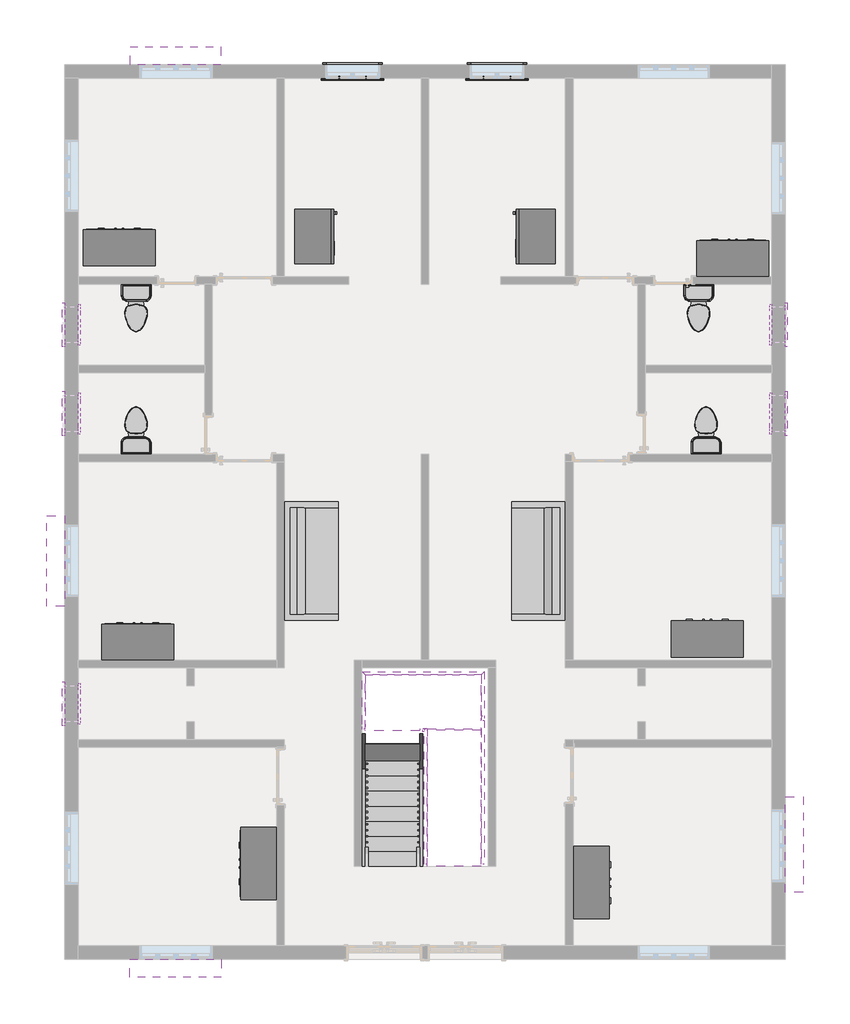
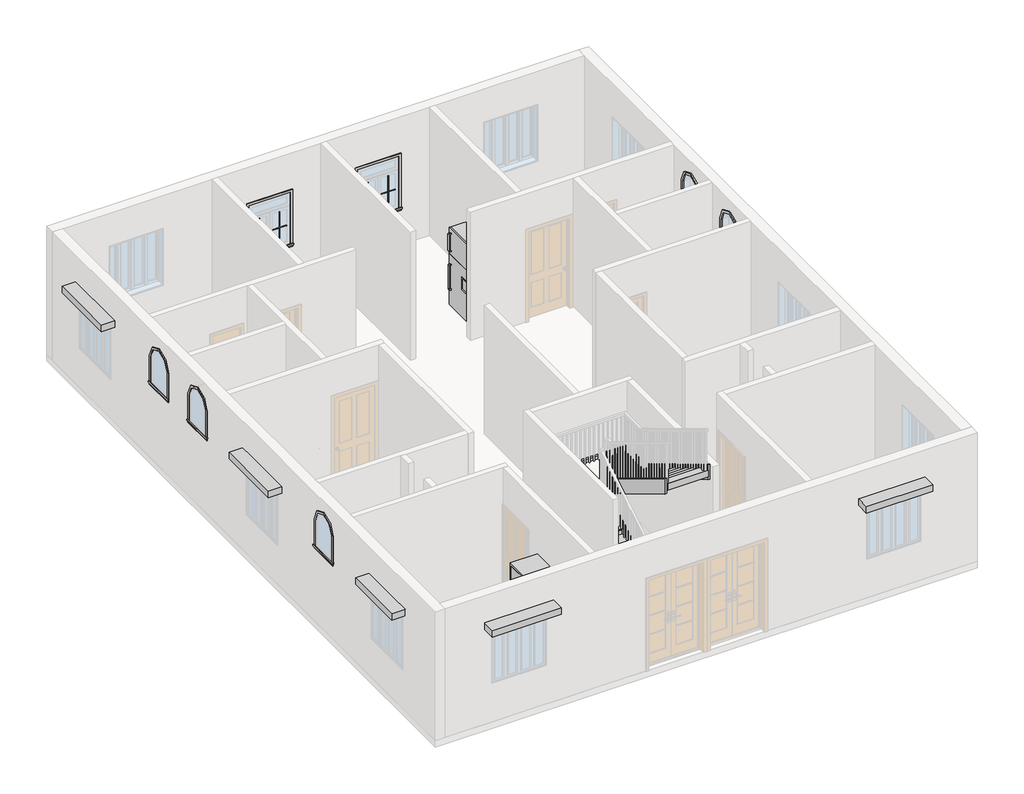
# One storey, part 4 of 4: 22 proxies, 10 furniture elements, 8 members, 4 flow terminals, 2 stair flights, 1 slab.
"""IFC4 building model written with IfcOpenShell, lengths in millimetres."""

from ifc_helpers import new_model, si_unit, frame, origin, place, context, project, spatial, polyline, outline, extrude, faceted_brep, transform, mapped, element, save
from components import generic_models_1_generic_models_1_2a4bce15, generic_models_2_generic_models_2_71c639ae, generic_models_3_generic_models_3_01e5b337, generic_models_4_generic_models_4_21550f0b, muntin_pattern_2x2_muntin_pattern_2x2_d1c6e638, muntin_pattern_2x2_muntin_pattern_2x2_37b95fb2, trim_window_exterior_flat_with_sill_80371c4b, trim_window_exterior_flat_arch_top_tree_centered_with_sill_b3d54518, trim_window_interior_flat_picture_frame_c1dcbb6d, trim_window_interior_flat_arch_top_tree_centered_picture_1d59b3d4, toilet_domestic_3d_toilet_domestic_3d_ba6479b0, toilet_domestic_3d_toilet_domestic_3d_30431060, furniture_65fa61b5, furniture_3f4f9d7a, furniture_123_or_4_seats_couch_4554_e45b83ba, furniture_82e269c4, non_monolithic_landing_68493687, stair_flight_7beec1f7, stair_flight_0e2f1c24

model = new_model("IFC4")

# Units and contexts
model_context = context("Model", 3, world=origin())
ifc_project = project(units=[si_unit("LENGTHUNIT", "METRE", prefix="MILLI")], contexts=[model_context])

# Site, building, storey
site = spatial("IfcSite", under=ifc_project)
building = spatial("IfcBuilding", under=site)
storey = spatial("IfcBuildingStorey", under=building, Elevation=0.0)

# Proxies
placement = place(None, origin())
generic_models_1_generic_models_1_shape = generic_models_1_generic_models_1_2a4bce15(model_context)
element("IfcBuildingElementProxy", 1, Name="Generic Models 1 : Generic Models 1", ObjectType="Generic Models 1 : Generic Models 1", at=placement, inside=storey, context=model_context, shape_type="MappedRepresentation", body=[
    mapped(generic_models_1_generic_models_1_shape, transform((0.0, 0.0, 0.0), x_axis=(1.0, 0.0, 0.0), y_axis=(0.0, 1.0, 0.0), z_axis=(0.0, 0.0, 1.0))),
])
generic_models_2_generic_models_2_shape = generic_models_2_generic_models_2_71c639ae(model_context)
element("IfcBuildingElementProxy", 2, Name="Generic Models 2 : Generic Models 2", ObjectType="Generic Models 2 : Generic Models 2", at=placement, inside=storey, context=model_context, shape_type="MappedRepresentation", body=[
    mapped(generic_models_2_generic_models_2_shape, transform((0.0, 0.0, 0.0), x_axis=(1.0, 0.0, 0.0), y_axis=(0.0, 1.0, 0.0), z_axis=(0.0, 0.0, 1.0))),
])
generic_models_3_generic_models_3_shape = generic_models_3_generic_models_3_01e5b337(model_context)
element("IfcBuildingElementProxy", 3, Name="Generic Models 3 : Generic Models 3", ObjectType="Generic Models 3 : Generic Models 3", at=placement, inside=storey, context=model_context, shape_type="MappedRepresentation", body=[
    mapped(generic_models_3_generic_models_3_shape, transform((0.0, 0.0, 0.0), x_axis=(1.0, 0.0, 0.0), y_axis=(0.0, 1.0, 0.0), z_axis=(0.0, 0.0, 1.0))),
])
generic_models_4_generic_models_4_shape = generic_models_4_generic_models_4_21550f0b(model_context)
element("IfcBuildingElementProxy", 4, Name="Generic Models 4 : Generic Models 4", ObjectType="Generic Models 4 : Generic Models 4", at=placement, inside=storey, context=model_context, shape_type="MappedRepresentation", body=[
    mapped(generic_models_4_generic_models_4_shape, transform((0.0, 0.0, 0.0), x_axis=(1.0, 0.0, 0.0), y_axis=(0.0, 1.0, 0.0), z_axis=(0.0, 0.0, 1.0))),
])
muntin_pattern_2x2_muntin_pattern_2x2_shape = muntin_pattern_2x2_muntin_pattern_2x2_d1c6e638(model_context)
element("IfcBuildingElementProxy", 5, Name="Muntin Pattern_2x2 : Muntin Pattern_2x2", ObjectType="Muntin Pattern_2x2 : Muntin Pattern_2x2", at=placement, inside=storey, context=model_context, shape_type="MappedRepresentation", body=[
    mapped(muntin_pattern_2x2_muntin_pattern_2x2_shape, transform((-10531.1646954, 8361.6522103, 984.25), x_axis=(-1.0, 0.0, 0.0), y_axis=(0.0, -1.0, 0.0), z_axis=(0.0, 0.0, 1.0))),
])
element("IfcBuildingElementProxy", 6, Name="Muntin Pattern_2x2 : Muntin Pattern_2x2", ObjectType="Muntin Pattern_2x2 : Muntin Pattern_2x2", at=placement, inside=storey, context=model_context, shape_type="MappedRepresentation", body=[
    mapped(muntin_pattern_2x2_muntin_pattern_2x2_shape, transform((-8092.7646954, 8361.6522103, 984.25), x_axis=(-1.0, 0.0, 0.0), y_axis=(0.0, -1.0, 0.0), z_axis=(0.0, 0.0, 1.0))),
])
muntin_pattern_2x2_muntin_pattern_2x2_2_shape = muntin_pattern_2x2_muntin_pattern_2x2_37b95fb2(model_context)
element("IfcBuildingElementProxy", 7, Name="Muntin Pattern_2x2 : Muntin Pattern_2x2", ObjectType="Muntin Pattern_2x2 : Muntin Pattern_2x2", at=placement, inside=storey, context=model_context, shape_type="MappedRepresentation", body=[
    mapped(muntin_pattern_2x2_muntin_pattern_2x2_2_shape, transform((-10985.1896954, 8361.6522103, 984.25), x_axis=(1.0, 0.0, 0.0), y_axis=(0.0, 1.0, 0.0), z_axis=(0.0, 0.0, 1.0))),
])
element("IfcBuildingElementProxy", 8, Name="Muntin Pattern_2x2 : Muntin Pattern_2x2", ObjectType="Muntin Pattern_2x2 : Muntin Pattern_2x2", at=placement, inside=storey, context=model_context, shape_type="MappedRepresentation", body=[
    mapped(muntin_pattern_2x2_muntin_pattern_2x2_2_shape, transform((-8546.7896954, 8361.6522103, 984.25), x_axis=(1.0, 0.0, 0.0), y_axis=(0.0, 1.0, 0.0), z_axis=(0.0, 0.0, 1.0))),
])
trim_window_exterior_flat_with_sill_shape = trim_window_exterior_flat_with_sill_80371c4b(model_context)
element("IfcBuildingElementProxy", 9, Name="Trim-Window-Exterior-Flat : with Sill", ObjectType="Trim-Window-Exterior-Flat : with Sill", at=placement, inside=storey, context=model_context, shape_type="MappedRepresentation", body=[
    mapped(trim_window_exterior_flat_with_sill_shape, transform((-10758.1771954, 8352.1272103, 2133.6), x_axis=(-1.0, 0.0, 0.0), y_axis=(0.0, 0.0, -1.0), z_axis=(0.0, -1.0, 0.0))),
])
element("IfcBuildingElementProxy", 10, Name="Trim-Window-Exterior-Flat : with Sill", ObjectType="Trim-Window-Exterior-Flat : with Sill", at=placement, inside=storey, context=model_context, shape_type="MappedRepresentation", body=[
    mapped(trim_window_exterior_flat_with_sill_shape, transform((-8319.7771954, 8352.1272103, 2133.6), x_axis=(-1.0, 0.0, 0.0), y_axis=(0.0, 0.0, -1.0), z_axis=(0.0, -1.0, 0.0))),
])
trim_window_exterior_flat_arch_top_tree_centered_with_sill_shape = trim_window_exterior_flat_arch_top_tree_centered_with_sill_b3d54518(model_context)
element("IfcBuildingElementProxy", 11, Name="Trim-Window-Exterior-Flat-Arch-Top-Tree_Centered : with Sill", ObjectType="Trim-Window-Exterior-Flat-Arch-Top-Tree_Centered : with Sill", at=placement, inside=storey, context=model_context, shape_type="MappedRepresentation", body=[
    mapped(trim_window_exterior_flat_arch_top_tree_centered_with_sill_shape, transform((-15623.8646954, -2214.2727897, 2743.2), x_axis=(0.0, -1.0, 0.0), y_axis=(0.0, 0.0, 1.0), z_axis=(-1.0, 0.0, 0.0))),
])
element("IfcBuildingElementProxy", 12, Name="Trim-Window-Exterior-Flat-Arch-Top-Tree_Centered : with Sill", ObjectType="Trim-Window-Exterior-Flat-Arch-Top-Tree_Centered : with Sill", at=placement, inside=storey, context=model_context, shape_type="MappedRepresentation", body=[
    mapped(trim_window_exterior_flat_arch_top_tree_centered_with_sill_shape, transform((-3455.6771954, 2688.1919086, 2743.2), x_axis=(0.0, 1.0, 0.0), y_axis=(0.0, 0.0, 1.0), z_axis=(1.0, 0.0, 0.0))),
])
element("IfcBuildingElementProxy", 13, Name="Trim-Window-Exterior-Flat-Arch-Top-Tree_Centered : with Sill", ObjectType="Trim-Window-Exterior-Flat-Arch-Top-Tree_Centered : with Sill", at=placement, inside=storey, context=model_context, shape_type="MappedRepresentation", body=[
    mapped(trim_window_exterior_flat_arch_top_tree_centered_with_sill_shape, transform((-3455.6771954, 4186.5272103, 2743.2), x_axis=(0.0, 1.0, 0.0), y_axis=(0.0, 0.0, 1.0), z_axis=(1.0, 0.0, 0.0))),
])
element("IfcBuildingElementProxy", 14, Name="Trim-Window-Exterior-Flat-Arch-Top-Tree_Centered : with Sill", ObjectType="Trim-Window-Exterior-Flat-Arch-Top-Tree_Centered : with Sill", at=placement, inside=storey, context=model_context, shape_type="MappedRepresentation", body=[
    mapped(trim_window_exterior_flat_arch_top_tree_centered_with_sill_shape, transform((-15623.8646954, 2688.1919086, 2743.2), x_axis=(0.0, -1.0, 0.0), y_axis=(0.0, 0.0, 1.0), z_axis=(-1.0, 0.0, 0.0))),
])
element("IfcBuildingElementProxy", 15, Name="Trim-Window-Exterior-Flat-Arch-Top-Tree_Centered : with Sill", ObjectType="Trim-Window-Exterior-Flat-Arch-Top-Tree_Centered : with Sill", at=placement, inside=storey, context=model_context, shape_type="MappedRepresentation", body=[
    mapped(trim_window_exterior_flat_arch_top_tree_centered_with_sill_shape, transform((-15623.8646954, 4186.5272103, 2743.2), x_axis=(0.0, -1.0, 0.0), y_axis=(0.0, 0.0, 1.0), z_axis=(-1.0, 0.0, 0.0))),
])
trim_window_interior_flat_picture_frame_shape = trim_window_interior_flat_picture_frame_c1dcbb6d(model_context)
element("IfcBuildingElementProxy", 16, Name="Trim-Window-Interior-Flat : Picture Frame", ObjectType="Trim-Window-Interior-Flat : Picture Frame", at=placement, inside=storey, context=model_context, shape_type="MappedRepresentation", body=[
    mapped(trim_window_interior_flat_picture_frame_shape, transform((-10758.1771954, 8580.7272103, 2133.6), x_axis=(1.0, 0.0, 0.0), y_axis=(0.0, 0.0, -1.0), z_axis=(0.0, 1.0, 0.0))),
])
element("IfcBuildingElementProxy", 17, Name="Trim-Window-Interior-Flat : Picture Frame", ObjectType="Trim-Window-Interior-Flat : Picture Frame", at=placement, inside=storey, context=model_context, shape_type="MappedRepresentation", body=[
    mapped(trim_window_interior_flat_picture_frame_shape, transform((-8319.7771954, 8580.7272103, 2133.6), x_axis=(1.0, 0.0, 0.0), y_axis=(0.0, 0.0, -1.0), z_axis=(0.0, 1.0, 0.0))),
])
trim_window_interior_flat_arch_top_tree_centered_picture_shape = trim_window_interior_flat_arch_top_tree_centered_picture_1d59b3d4(model_context)
element("IfcBuildingElementProxy", 18, Name="Trim-Window-Interior-Flat-Arch-Top-Tree_Centered : Picture Frame", ObjectType="Trim-Window-Interior-Flat-Arch-Top-Tree_Centered : Picture Frame", at=placement, inside=storey, context=model_context, shape_type="MappedRepresentation", body=[
    mapped(trim_window_interior_flat_arch_top_tree_centered_picture_shape, transform((-15395.2646954, -2214.2727897, 2743.2), x_axis=(0.0, 1.0, 0.0), y_axis=(0.0, 0.0, 1.0), z_axis=(1.0, 0.0, 0.0))),
])
element("IfcBuildingElementProxy", 19, Name="Trim-Window-Interior-Flat-Arch-Top-Tree_Centered : Picture Frame", ObjectType="Trim-Window-Interior-Flat-Arch-Top-Tree_Centered : Picture Frame", at=placement, inside=storey, context=model_context, shape_type="MappedRepresentation", body=[
    mapped(trim_window_interior_flat_arch_top_tree_centered_picture_shape, transform((-3684.2771954, 2688.1919086, 2743.2), x_axis=(0.0, -1.0, 0.0), y_axis=(0.0, 0.0, 1.0), z_axis=(-1.0, 0.0, 0.0))),
])
element("IfcBuildingElementProxy", 20, Name="Trim-Window-Interior-Flat-Arch-Top-Tree_Centered : Picture Frame", ObjectType="Trim-Window-Interior-Flat-Arch-Top-Tree_Centered : Picture Frame", at=placement, inside=storey, context=model_context, shape_type="MappedRepresentation", body=[
    mapped(trim_window_interior_flat_arch_top_tree_centered_picture_shape, transform((-3684.2771954, 4186.5272103, 2743.2), x_axis=(0.0, -1.0, 0.0), y_axis=(0.0, 0.0, 1.0), z_axis=(-1.0, 0.0, 0.0))),
])
element("IfcBuildingElementProxy", 21, Name="Trim-Window-Interior-Flat-Arch-Top-Tree_Centered : Picture Frame", ObjectType="Trim-Window-Interior-Flat-Arch-Top-Tree_Centered : Picture Frame", at=placement, inside=storey, context=model_context, shape_type="MappedRepresentation", body=[
    mapped(trim_window_interior_flat_arch_top_tree_centered_picture_shape, transform((-15395.2646954, 2688.1919086, 2743.2), x_axis=(0.0, 1.0, 0.0), y_axis=(0.0, 0.0, 1.0), z_axis=(1.0, 0.0, 0.0))),
])
element("IfcBuildingElementProxy", 22, Name="Trim-Window-Interior-Flat-Arch-Top-Tree_Centered : Picture Frame", ObjectType="Trim-Window-Interior-Flat-Arch-Top-Tree_Centered : Picture Frame", at=placement, inside=storey, context=model_context, shape_type="MappedRepresentation", body=[
    mapped(trim_window_interior_flat_arch_top_tree_centered_picture_shape, transform((-15395.2646954, 4186.5272103, 2743.2), x_axis=(0.0, 1.0, 0.0), y_axis=(0.0, 0.0, 1.0), z_axis=(1.0, 0.0, 0.0))),
])

# Flow terminals
toilet_domestic_3d_toilet_domestic_3d_shape = toilet_domestic_3d_toilet_domestic_3d_ba6479b0(model_context)
toilet_domestic_3d_toilet_domestic_3d_2_shape = toilet_domestic_3d_toilet_domestic_3d_30431060(model_context)
element("IfcFlowTerminal", 23, ObjectType="Toilet-Domestic-3D : Toilet-Domestic-3D", at=placement, inside=storey, context=model_context, shape_type="MappedRepresentation", body=[
    mapped(toilet_domestic_3d_toilet_domestic_3d_shape, transform((-14415.7771954, 4377.631183, 0.0), x_axis=(1.0, 0.0, 0.0), y_axis=(0.0, 1.0, 0.0), z_axis=(0.0, 0.0, 1.0))),
    mapped(toilet_domestic_3d_toilet_domestic_3d_2_shape, transform((-14415.7771954, 4377.631183, 0.0), x_axis=(1.0, 0.0, 0.0), y_axis=(0.0, 1.0, 0.0), z_axis=(0.0, 0.0, 1.0))),
])
element("IfcFlowTerminal", 24, ObjectType="Toilet-Domestic-3D : Toilet-Domestic-3D", at=placement, inside=storey, context=model_context, shape_type="MappedRepresentation", body=[
    mapped(toilet_domestic_3d_toilet_domestic_3d_shape, transform((-14417.3646954, 2497.3526342, 0.0), x_axis=(-1.0, 0.0, 0.0), y_axis=(0.0, -1.0, 0.0), z_axis=(0.0, 0.0, 1.0))),
    mapped(toilet_domestic_3d_toilet_domestic_3d_2_shape, transform((-14417.3646954, 2497.3526342, 0.0), x_axis=(-1.0, 0.0, 0.0), y_axis=(0.0, -1.0, 0.0), z_axis=(0.0, 0.0, 1.0))),
])
element("IfcFlowTerminal", 25, ObjectType="Toilet-Domestic-3D : Toilet-Domestic-3D", at=placement, inside=storey, context=model_context, shape_type="MappedRepresentation", body=[
    mapped(toilet_domestic_3d_toilet_domestic_3d_shape, transform((-4789.1771954, 2497.3526342, 0.0), x_axis=(-1.0, 0.0, 0.0), y_axis=(0.0, -1.0, 0.0), z_axis=(0.0, 0.0, 1.0))),
    mapped(toilet_domestic_3d_toilet_domestic_3d_2_shape, transform((-4789.1771954, 2497.3526342, 0.0), x_axis=(-1.0, 0.0, 0.0), y_axis=(0.0, -1.0, 0.0), z_axis=(0.0, 0.0, 1.0))),
])
element("IfcFlowTerminal", 26, ObjectType="Toilet-Domestic-3D : Toilet-Domestic-3D", at=placement, inside=storey, context=model_context, shape_type="MappedRepresentation", body=[
    mapped(toilet_domestic_3d_toilet_domestic_3d_shape, transform((-4916.1771954, 4377.631183, 0.0), x_axis=(1.0, 0.0, 0.0), y_axis=(0.0, 1.0, 0.0), z_axis=(0.0, 0.0, 1.0))),
    mapped(toilet_domestic_3d_toilet_domestic_3d_2_shape, transform((-4916.1771954, 4377.631183, 0.0), x_axis=(1.0, 0.0, 0.0), y_axis=(0.0, 1.0, 0.0), z_axis=(0.0, 0.0, 1.0))),
])

# Furniture
furniture_shape = furniture_65fa61b5(model_context)
element("IfcFurniture", 27, at=placement, inside=storey, context=model_context, shape_type="MappedRepresentation", body=[
    mapped(furniture_shape, transform((-11740.80602, 6289.078474, 0.0), x_axis=(0.0, 1.0, 0.0), y_axis=(-1.0, 0.0, 0.0), z_axis=(0.0, 0.0, 1.0))),
])
furniture_2_shape = furniture_3f4f9d7a(model_context)
element("IfcFurniture", 28, at=placement, inside=storey, context=model_context, shape_type="MappedRepresentation", body=[
    mapped(furniture_2_shape, transform((-7338.7358708, 6289.078474, 0.0), x_axis=(0.0, 1.0, 0.0), y_axis=(-1.0, 0.0, 0.0), z_axis=(0.0, 0.0, 1.0))),
])
furniture_123_or_4_seats_couch_4554_shape = furniture_123_or_4_seats_couch_4554_e45b83ba(model_context)
element("IfcFurniture", 29, ObjectType="123_or_4_seats_couch_4554", at=placement, inside=storey, context=model_context, shape_type="MappedRepresentation", body=[
    mapped(furniture_123_or_4_seats_couch_4554_shape, transform((-11913.8771954, 122.7919086, 0.0), x_axis=(8.148770547222739e-11, 1.0, 0.0), y_axis=(-1.0, 8.148770547222739e-11, 0.0), z_axis=(0.0, 0.0, 1.0))),
])
element("IfcFurniture", 30, ObjectType="123_or_4_seats_couch_4554", at=placement, inside=storey, context=model_context, shape_type="MappedRepresentation", body=[
    mapped(furniture_123_or_4_seats_couch_4554_shape, transform((-7164.0771954, 275.1919086, 0.0), x_axis=(0.0, -1.0, 0.0), y_axis=(1.0, 0.0, 0.0), z_axis=(0.0, 0.0, 1.0))),
])
furniture_3_shape = furniture_82e269c4(model_context)
element("IfcFurniture", 31, ObjectType="Wardrobe : 48\" x 72\" x 24\"", at=placement, inside=storey, context=model_context, shape_type="MappedRepresentation", body=[
    mapped(furniture_3_shape, transform((-14969.1544857, 4905.0525787, 0.0), x_axis=(-1.0, 0.0, 0.0), y_axis=(0.0, -1.0, 0.0), z_axis=(0.0, 0.0, 1.0))),
])
element("IfcFurniture", 32, ObjectType="Wardrobe : 48\" x 72\" x 24\"", at=placement, inside=storey, context=model_context, shape_type="MappedRepresentation", body=[
    mapped(furniture_3_shape, transform((-4609.4240791, 4720.3884008, 0.0), x_axis=(-1.0, 0.0, 0.0), y_axis=(0.0, -1.0, 0.0), z_axis=(0.0, 0.0, 1.0))),
])
element("IfcFurniture", 33, ObjectType="Wardrobe : 48\" x 72\" x 24\"", at=placement, inside=storey, context=model_context, shape_type="MappedRepresentation", body=[
    mapped(furniture_3_shape, transform((-14654.9354475, -1756.6115992, 0.0), x_axis=(-1.0, 0.0, 0.0), y_axis=(0.0, -1.0, 0.0), z_axis=(0.0, 0.0, 1.0))),
])
element("IfcFurniture", 34, ObjectType="Wardrobe : 48\" x 72\" x 24\"", at=placement, inside=storey, context=model_context, shape_type="MappedRepresentation", body=[
    mapped(furniture_3_shape, transform((-5037.6875981, -1704.33178, 0.0), x_axis=(-1.0, 0.0, 0.0), y_axis=(0.0, -1.0, 0.0), z_axis=(0.0, 0.0, 1.0))),
])
element("IfcFurniture", 35, ObjectType="Wardrobe : 48\" x 72\" x 24\"", at=placement, inside=storey, context=model_context, shape_type="MappedRepresentation", body=[
    mapped(furniture_3_shape, transform((-7316.016005, -4965.0574511, 0.0), x_axis=(0.0, 1.0, 0.0), y_axis=(-1.0, 0.0, 0.0), z_axis=(0.0, 0.0, 1.0))),
])
element("IfcFurniture", 36, ObjectType="Wardrobe : 48\" x 72\" x 24\"", at=placement, inside=storey, context=model_context, shape_type="MappedRepresentation", body=[
    mapped(furniture_3_shape, transform((-11761.9383858, -5181.4279362, 0.0), x_axis=(0.0, -1.0, 0.0), y_axis=(1.0, 0.0, 0.0), z_axis=(0.0, 0.0, 1.0))),
])

# Members
element("IfcMember", 37, ObjectType="Stringer - 2\" Width", at=placement, inside=storey, context=model_context, shape_type="SweptSolid", body=[
    extrude(outline(polyline([(-4957.4727897, 0.0), (-4957.4727897, 211.5517384), (-2643.0590204, 1600.2), (-2558.6343079, 1295.4), (-4717.6343079, 0.0), (-4957.4727897, 0.0)])), frame((-10593.0771954, 0.0, 0.0), z_axis=(1.0, 0.0, 0.0), x_axis=(0.0, 1.0, 0.0)), (0.0, 0.0, 1.0), 50.8),
])
element("IfcMember", 38, ObjectType="Stringer - 2\" Width", at=placement, inside=storey, context=model_context, shape_type="SweptSolid", body=[
    extrude(outline(polyline([(-4957.4727897, 0.0), (-4957.4727897, 211.5517384), (-2643.0590204, 1600.2), (-2639.7227897, 1600.2), (-2639.7227897, 1246.7469109), (-4717.6343079, 0.0), (-4957.4727897, 0.0)])), frame((-9627.8771954, 0.0, 0.0), z_axis=(1.0, 0.0, 0.0), x_axis=(0.0, 1.0, 0.0)), (0.0, 0.0, 1.0), 50.8),
])
element("IfcMember", 39, ObjectType="Stringer - 2\" Width", at=placement, inside=storey, context=model_context, shape_type="SweptSolid", body=[
    extrude(outline(polyline([(-2414.1365589, 1600.2), (-2498.5612714, 1295.4), (-4925.7227897, 2751.6969109), (-4925.7227897, 3107.1517384), (-2414.1365589, 1600.2)])), frame((-8586.4771954, 0.0, 0.0), z_axis=(1.0, 0.0, 0.0), x_axis=(0.0, 1.0, 0.0)), (0.0, 0.0, 1.0), 50.8),
])
element("IfcMember", 40, ObjectType="Stringer - 2\" Width", at=placement, inside=storey, context=model_context, shape_type="SweptSolid", body=[
    extrude(outline(polyline([(-2639.7227897, 1735.5517384), (-2639.7227897, 1380.0969109), (-4925.7227897, 2751.6969109), (-4925.7227897, 3107.1517384), (-2639.7227897, 1735.5517384)])), frame((-9551.6771954, 0.0, 0.0), z_axis=(1.0, 0.0, 0.0), x_axis=(0.0, 1.0, 0.0)), (0.0, 0.0, 1.0), 50.8),
])
element("IfcMember", 41, ObjectType="Stringer - 2\" Width", at=placement, inside=storey, context=model_context, shape_type="Brep", body=[
    faceted_brep([(-8586.4771954, -2414.1365589, 1600.2), (-8535.6771954, -2414.1365589, 1600.2), (-8535.6771954, -1674.5227897, 1600.2), (-8586.4771954, -1725.3227897, 1600.2), (-8586.4771954, -2498.5612714, 1295.4), (-8586.4771954, -1725.3227897, 1295.4), (-8535.6771954, -2498.5612714, 1295.4), (-8535.6771954, -1674.5227897, 1295.4)], [[[0, 1, 2, 3]], [[4, 0, 3, 5]], [[6, 4, 5, 7]], [[1, 6, 7, 2]], [[1, 0, 4, 6]], [[2, 7, 5, 3]]]),
])
element("IfcMember", 42, ObjectType="Stringer - 2\" Width", at=placement, inside=storey, context=model_context, shape_type="SweptSolid", body=[
    extrude(outline(polyline([(-8535.6771954, -1674.5227897), (-8586.4771954, -1725.3227897), (-10542.2771954, -1725.3227897), (-10593.0771954, -1674.5227897), (-8535.6771954, -1674.5227897)])), frame((0.0, 0.0, 1295.4), z_axis=(0.0, 0.0, 1.0), x_axis=(1.0, 0.0, 0.0)), (0.0, 0.0, 1.0), 304.8),
])
element("IfcMember", 43, ObjectType="Stringer - 2\" Width", at=placement, inside=storey, context=model_context, shape_type="Brep", body=[
    faceted_brep([(-10542.2771954, -1725.3227897, 1600.2), (-10593.0771954, -1674.5227897, 1600.2), (-10593.0771954, -2643.0590204, 1600.2), (-10542.2771954, -2643.0590204, 1600.2), (-10542.2771954, -1725.3227897, 1295.4), (-10542.2771954, -2558.6343079, 1295.4), (-10593.0771954, -1674.5227897, 1295.4), (-10593.0771954, -2558.6343079, 1295.4)], [[[0, 1, 2, 3]], [[4, 0, 3, 5]], [[6, 4, 5, 7]], [[1, 6, 7, 2]], [[1, 0, 4, 6]], [[2, 7, 5, 3]]]),
])
element("IfcMember", 44, ObjectType="Stringer - 2\" Width", at=placement, inside=storey, context=model_context, shape_type="SweptSolid", body=[
    extrude(outline(polyline([(-9577.0771954, -2690.5227897), (-9577.0771954, -2639.7227897), (-9551.6771954, -2639.7227897), (-9551.6771954, -2690.5227897), (-9577.0771954, -2690.5227897)])), frame((0.0, 0.0, 1295.4), z_axis=(0.0, 0.0, 1.0), x_axis=(1.0, 0.0, 0.0)), (0.0, 0.0, 1.0), 304.8),
])

# Slab
non_monolithic_landing_shape = non_monolithic_landing_68493687(model_context)
element("IfcSlab", 45, ObjectType="Non-Monolithic Landing", at=placement, inside=storey, context=model_context, shape_type="MappedRepresentation", body=[
    mapped(non_monolithic_landing_shape, transform((0.0, 0.0, 0.0), x_axis=(1.0, 0.0, 0.0), y_axis=(0.0, 1.0, 0.0), z_axis=(0.0, 0.0, 1.0))),
])

# Stair flights
stair_flight_shape = stair_flight_7beec1f7(model_context)
element("IfcStairFlight", 46, ObjectType="2\" Tread 1\" Nosing 1/4\" Riser", at=placement, inside=storey, context=model_context, shape_type="MappedRepresentation", body=[
    mapped(stair_flight_shape, transform((0.0, 0.0, 0.0), x_axis=(1.0, 0.0, 0.0), y_axis=(0.0, 1.0, 0.0), z_axis=(0.0, 0.0, 1.0))),
])
stair_flight_2_shape = stair_flight_0e2f1c24(model_context)
element("IfcStairFlight", 47, ObjectType="2\" Tread 1\" Nosing 1/4\" Riser", at=placement, inside=storey, context=model_context, shape_type="MappedRepresentation", body=[
    mapped(stair_flight_2_shape, transform((0.0, 0.0, 0.0), x_axis=(1.0, 0.0, 0.0), y_axis=(0.0, 1.0, 0.0), z_axis=(0.0, 0.0, 1.0))),
])

save(model, "model.ifc")

# Revit data of these elements
# Type "Muntin Pattern_2x2 : Muntin Pattern_2x2"
#   Width [instance default] = 4' - 0"
#   Thickness = 0' - 0 1/2"
#   Height [instance default] = 4' - 0"
#   Distance = 0' - 0 3/4"
#   Interior Material [instance default] = none
#   Exterior Material [instance default] = none
#   Default Elevation = 0
# Type "Trim-Window-Exterior-Flat : with Sill"
#   Trim Width = 0' - 2 1/4"
#   Trim Thickness_Picture Frame = 0' - 1 1/4"
#   Trim Thickness_with Sill = 0' - 0 3/4"
#   Sill Thickness = 0' - 1 1/4"
#   Opening Width [instance default] = 2' - 0"
#   Opening Height [instance default] = 3' - 0"
#   Default Elevation = 4' - 0"
#   Sill = yes
#   Picture Frame = no
#   Trim Material [instance default] = none
# Type "Trim-Window-Exterior-Flat-Arch-Top-Tree_Centered : with Sill"
#   Trim Width = 0' - 2 1/4"
#   Trim Thickness_Picture Frame = 0' - 1 1/4"
#   Trim Thickness_with Sill = 0' - 0 3/4"
#   Sill Thickness = 0' - 1 1/4"
#   Opening Width [instance default] = 2' - 0"
#   Opening Height [instance default] = 3' - 0"
#   Default Elevation = 4' - 0"
#   Sill = yes
#   Picture Frame = no
#   Trim Material [instance default] = none
# Type "Trim-Window-Interior-Flat : Picture Frame"
#   Trim Thickness_Picture Frame = 0' - 1 1/4"
#   Trim Width = 0' - 2 1/4"
#   Trim Thickness_with Sill = 0' - 0 3/4"
#   Sill Thickness = 0' - 1 1/4"
#   Opening Width [instance default] = 2' - 0"
#   Opening Height [instance default] = 3' - 0"
#   Default Elevation = 4' - 0"
#   Sill = no
#   Picture Frame = yes
#   Trim Material [instance default] = none
# Type "Trim-Window-Interior-Flat-Arch-Top-Tree_Centered : Picture Frame"
#   Trim Thickness_Picture Frame = 0' - 1 1/4"
#   Trim Width = 0' - 2 1/4"
#   Trim Thickness_with Sill = 0' - 0 3/4"
#   Sill Thickness = 0' - 1 1/4"
#   Opening Width [instance default] = 2' - 0"
#   Opening Height [instance default] = 3' - 0"
#   Default Elevation = 4' - 0"
#   Sill = no
#   Picture Frame = yes
#   Trim Material [instance default] = none
# Type "Toilet-Domestic-3D : Toilet-Domestic-3D"
#   Assembly Code = "D2010110"
#   Toilet - Bowl/Basin Material = Porcelain, Linen
#   Toilet - Seat Material = Laminate, Linen, Matte
#   Default Elevation = 0
# Type
#   Default Elevation = 0
# Type "123_or_4_seats_couch_4554"
#   width = 6' - 6.74016"
#   seat height = 1' - 5.71654"
#   height = 2' - 5.92126"
#   depth = 2' - 11.82677"
#   arm height = 1' - 7.68504"
#   arm depth = 0' - 3.93701"
#   Total Seat Room = 5' - 10.86614"
#   Seat Width = 1' - 11.62205"
#   Seat Count = 3
#   Is Mark Visible = yes
#   seat material = Sofa seat
#   arm material = Sofa arm
#   Default Elevation = 0
#   Assembly Code = ""
# Type "Wardrobe : 48\" x 72\" x 24\""
#   Assembly Code = "E2020200"
#   Depth = 2' - 0"
#   Height = 6' - 0"
#   Width = 4' - 0"
#   Material = Wood - Mahogany
#   Default Elevation = 0
# Element 1 (IfcBuildingElementProxy, "Generic Models 1 : Generic Models 1")
#   Phase Created = New Construction
# Element 2 (IfcBuildingElementProxy, "Generic Models 2 : Generic Models 2")
#   Phase Created = New Construction
# Element 3 (IfcBuildingElementProxy, "Generic Models 3 : Generic Models 3")
#   Phase Created = New Construction
# Element 4 (IfcBuildingElementProxy, "Generic Models 4 : Generic Models 4")
#   Phase Created = New Construction
# Elements 5, 6, 7, 8 (IfcBuildingElementProxy, "Muntin Pattern_2x2 : Muntin Pattern_2x2")
#   Width = 1' - 0 5/8"
#   Height = 2' - 6 1/2"
#   Interior Material = Wood - Stained
#   Exterior Material = Clad - White
#   Phase Created = New Construction
#   Materials on its faces: "Clad - White", "Wood - Stained"
# Elements 9, 10 (IfcBuildingElementProxy, "Trim-Window-Exterior-Flat : with Sill")
#   Opening Width = 3' - 0"
#   Opening Height = 4' - 0"
#   Trim Material = Clad - White
#   Phase Created = New Construction
#   Materials on its faces: "Clad - White"
# Elements 11, 12, 13, 14, 15 (IfcBuildingElementProxy, "Trim-Window-Exterior-Flat-Arch-Top-Tree_Centered : with Sill")
#   Opening Width = 2' - 0"
#   Opening Height = 3' - 0"
#   Trim Material = Clad - White
#   Phase Created = New Construction
#   Materials on its faces: "Clad - White"
# Elements 16, 17 (IfcBuildingElementProxy, "Trim-Window-Interior-Flat : Picture Frame")
#   Opening Width = 3' - 0"
#   Opening Height = 4' - 0"
#   Trim Material = Wood - Stained
#   Phase Created = New Construction
#   Materials on its faces: "Wood - Stained"
# Elements 18, 19, 20, 21, 22 (IfcBuildingElementProxy, "Trim-Window-Interior-Flat-Arch-Top-Tree_Centered : Picture Frame")
#   Opening Width = 2' - 0"
#   Opening Height = 3' - 0"
#   Trim Material = Wood - Stained
#   Phase Created = New Construction
#   Materials on its faces: "Wood - Stained"
# Element 23 (IfcFlowTerminal, "Toilet-Domestic-3D : Toilet-Domestic-3D")
#   Mark = "1"
#   Phase Created = New Construction
#   Materials on its faces: "Porcelain, Linen", "Laminate, Linen, Matte"
# Element 24 (IfcFlowTerminal, "Toilet-Domestic-3D : Toilet-Domestic-3D")
#   Mark = "2"
#   Phase Created = New Construction
#   Materials on its faces: "Porcelain, Linen", "Laminate, Linen, Matte"
# Element 25 (IfcFlowTerminal, "Toilet-Domestic-3D : Toilet-Domestic-3D")
#   Mark = "3"
#   Phase Created = New Construction
#   Materials on its faces: "Porcelain, Linen", "Laminate, Linen, Matte"
# Element 26 (IfcFlowTerminal, "Toilet-Domestic-3D : Toilet-Domestic-3D")
#   Mark = "4"
#   Phase Created = New Construction
#   Materials on its faces: "Porcelain, Linen", "Laminate, Linen, Matte"
# Elements 27, 28 (IfcFurniture)
#   Phase Created = New Construction
#   Materials on its faces: "Default", "Default 3", "Default 2"
# Elements 29, 30 (IfcFurniture, "123_or_4_seats_couch_4554")
#   Phase Created = New Construction
#   Materials on its faces: "Sofa seat", "Sofa arm"
# Elements 31, 32, 33, 34, 35, 36 (IfcFurniture, "Wardrobe : 48\" x 72\" x 24\"")
#   Phase Created = New Construction
#   Materials on its faces: "Wood - Mahogany"
# Elements 37, 38, 39, 40, 41, 42, 43, 44 (IfcMember, "Stringer - 2\" Width")
#   Phase Created = New Construction
# Element 45 (IfcSlab, "Non-Monolithic Landing")
#   Phase Created = New Construction
# Element 46 (IfcStairFlight, "2\" Tread 1\" Nosing 1/4\" Riser")
#   Phase Created = New Construction
# Element 47 (IfcStairFlight, "2\" Tread 1\" Nosing 1/4\" Riser")
#   Phase Created = New Construction
#   Materials on its faces: "Porcelain, Linen"
# Materials
#   "Porcelain, Linen": class "Ceramic", colour RGB 249 239 230, transparency 0, Description = "Porcelain, linen", Cost = 0
#   "Laminate, Linen, Matte": class "Plastic", colour RGB 249 239 230, transparency 0, Description = "Plastic Laminate - Linen, Matte", Cost = 0
#   "Sofa seat": colour RGB 247 247 239, transparency 0
#   "Sofa arm": colour RGB 247 247 239, transparency 0
#   "Wood - Mahogany": colour RGB 138 86 45, transparency 0
#   "Clad - White": class "Wood", colour RGB 242 242 238, transparency 0, Cost = 0
#   "Wood - Stained": class "Wood", colour RGB 224 178 126, transparency 0, Cost = 0
#   "Default": colour RGB 127 127 127, transparency 0, Cost = 0
#   "Default 3": class "Glass", colour RGB 127 127 127, transparency 0
#   "Default 2": class "Plastic", colour RGB 127 127 127, transparency 0
